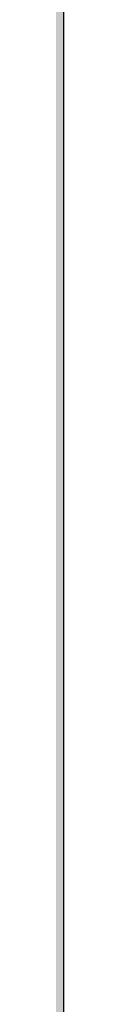
# Model space of a CAD drawing. Units: inches. Extents: x 2091 to 2899, y 967 to 2217.
# Tile 66 of 256: x 2212.1436 to 2212.1443, y 1100.4988 to 1101.1654. Entities that reach past the tile are written whole.
import ezdxf

# ---------------------------------------------------------------- set-up
doc = ezdxf.new("R2010")
doc.units = ezdxf.units.IN
doc.layers.add('A-ANNO-DIMS', color=2, linetype='Continuous', lineweight=18)
doc.layers.add('A-WALL-PATT', color=141, linetype='Continuous', lineweight=13, true_color=0xadddf7)
doc.styles.get("Standard").update_dxf_attribs({"font": 'arial.ttf'})
doc.dimstyles.new('ISO-25', dxfattribs={"dimtxt": 4, "dimasz": 4, "dimexe": 1.25, "dimexo": 0.625, "dimtad": 1, "dimdec": 0, "dimlunit": 3, "dimtxsty": 'Standard', "dimcen": 2.5, "dimadec": 0, "dimazin": 0, "dimtfac": 1, "dimtdec": 0, "dimtmove": 0, "dimatfit": 3, "dimfxl": 1, "dimarcsym": 0})

# ---------------------------------------------------------------- blocks, each defined once
blk = doc.blocks.new('*D71')
at = {"layer": 'A-ANNO-DIMS', "color": 0, "lineweight": -2, "transparency": 16777216}
for p, q in [((2212.1436, 1351.29406), (2212.1436, 969.4643)), ((2452.1436, 1351.29406), (2452.1436, 969.4643)), ((2216.1436, 970.7143), (2448.1436, 970.7143))]:
    blk.add_line(p, q, dxfattribs=at)
at = {"layer": 'A-ANNO-DIMS', "color": 0, "transparency": 16777216}
for points in [[(2216.1436, 971.38097), (2216.1436, 970.04764), (2212.1436, 970.7143)], [(2448.1436, 971.38097), (2448.1436, 970.04764), (2452.1436, 970.7143)]]:
    blk.add_solid(points, dxfattribs=at)
at = {"layer": 'Defpoints', "color": 0, "transparency": 16777216}
for p in [(2212.1436, 1351.91906), (2452.1436, 1351.91906), (2452.1436, 970.7143)]:
    blk.add_point(p, dxfattribs=at)
at = {"layer": 'A-ANNO-DIMS', "color": 0, "transparency": 16777216, "insert": (2332.1436, 973.38159), "char_height": 4, "attachment_point": 5}
blk.add_mtext('20\'-0"', dxfattribs=at)
blk = doc.blocks.new('*D75')
at = {"layer": 'A-ANNO-DIMS', "color": 0, "lineweight": -2, "transparency": 16777216}
for p, q in [((2212.1436, 1274.79406), (2212.1436, 969.4643)), ((2308.1436, 1274.79406), (2308.1436, 969.4643)), ((2216.1436, 970.7143), (2304.1436, 970.7143))]:
    blk.add_line(p, q, dxfattribs=at)
at = {"layer": 'A-ANNO-DIMS', "color": 0, "transparency": 16777216}
for points in [[(2216.1436, 971.38097), (2216.1436, 970.04764), (2212.1436, 970.7143)], [(2304.1436, 971.38097), (2304.1436, 970.04764), (2308.1436, 970.7143)]]:
    blk.add_solid(points, dxfattribs=at)
at = {"layer": 'Defpoints', "color": 0, "transparency": 16777216}
for p in [(2212.1436, 1275.41906), (2308.1436, 1275.41906), (2308.1436, 970.7143)]:
    blk.add_point(p, dxfattribs=at)
at = {"layer": 'A-ANNO-DIMS', "color": 0, "transparency": 16777216, "insert": (2260.1436, 973.38159), "char_height": 4, "attachment_point": 5}
blk.add_mtext('8\'-0"', dxfattribs=at)
blk = doc.blocks.new('*D91')
at = {"layer": 'A-ANNO-DIMS', "color": 0, "lineweight": -2, "transparency": 16777216}
for p, q in [((2211.65063, 1152.24706), (2098.31133, 1152.24706)), ((2099.56133, 1103.91906), (2099.56133, 1148.24706)), ((2211.5186, 1099.91906), (2098.31133, 1099.91906))]:
    blk.add_line(p, q, dxfattribs=at)
at = {"layer": 'A-ANNO-DIMS', "color": 0, "transparency": 16777216}
for points in [[(2098.89467, 1148.24706), (2100.228, 1148.24706), (2099.56133, 1152.24706)], [(2098.89467, 1103.91906), (2100.228, 1103.91906), (2099.56133, 1099.91906)]]:
    blk.add_solid(points, dxfattribs=at)
at = {"layer": 'Defpoints', "color": 0, "transparency": 16777216}
for p in [(2099.56133, 1152.24706), (2212.27563, 1152.24706), (2212.1436, 1099.91906)]:
    blk.add_point(p, dxfattribs=at)
at = {"layer": 'A-ANNO-DIMS', "color": 0, "transparency": 16777216, "insert": (2096.86812, 1126.08306), "char_height": 4, "attachment_point": 5, "rotation": 90}
blk.add_mtext('4\'-4 1/2"', dxfattribs=at)

msp = doc.modelspace()

# ---------------------------------------------------------------- hatches: boundary and pattern name
at = {"layer": 'A-WALL-PATT'}
h = msp.add_hatch(color=256, dxfattribs=at)
h.dxf.hatch_style = 1
h.paths.add_polyline_path([(2803.1436, 2050.91906), (2203.1436, 2050.91906), (2203.1436, 1090.91906), (2803.1436, 1090.91906)])
h.paths.add_polyline_path([(2635.79885, 1147.54046), (2674.52405, 1147.54046, 0.376086), (2678.52967, 1152.8802), (2678.52967, 1159.55647, 0.333335), (2674.52432, 1163.56185), (2674.52432, 1163.56185), (2674.52432, 1192.93439), (2635.80597, 1192.93439), (2597.08762, 1192.93439), (2597.08762, 1163.56185, 0.333335), (2593.08228, 1159.55647), (2593.08228, 1152.8802, 0.376086), (2597.08789, 1147.54046)], flags=0)
h.paths.add_polyline_path([(2436.01043, 1278.24078, 0.000483), (2435.95264, 1278.21503, -0.001328), (2435.93563, 1278.11169, -0.001711), (2436.11644, 1278.04076, 0.002185)], flags=0)
h.paths.add_polyline_path([(2794.1436, 1143.41906), (2794.1436, 1347.41906), (2543.37017, 1347.41906), (2543.37017, 1351.91906), (2794.1436, 1351.91906), (2794.1436, 1392.71355), (2793.9474, 1392.71355), (2793.9474, 1473.5369), (2794.1436, 1473.5369), (2794.1436, 1531.91906), (2650.1436, 1531.91906), (2650.1436, 1536.41906), (2794.1436, 1536.41906), (2794.1436, 1692.41906), (2609.37561, 1692.41906), (2609.37561, 1644.41906), (2604.87561, 1644.41906), (2604.87561, 1744.91906), (2609.37561, 1744.91906), (2609.37561, 1696.91906), (2794.1436, 1696.91906), (2794.1436, 1780.91906), (2609.6436, 1780.91906), (2493.87561, 1780.91906), (2493.87561, 1785.41906), (2609.6436, 1785.41906), (2794.1436, 1785.41906), (2794.1436, 1847.93882), (2793.95122, 1847.93882), (2793.95122, 1928.76217), (2794.1436, 1928.76217), (2794.1436, 1941.41906), (2614.1436, 1941.41906), (2614.1436, 1821.41906), (2609.6436, 1821.41906), (2609.6436, 1941.41906), (2392.1436, 1941.41906), (2392.1436, 1819.91906), (2387.6436, 1819.91906), (2387.6436, 1941.41906), (2212.1436, 1941.41906), (2212.1436, 1783.91906), (2392.1436, 1783.91906), (2392.1436, 1780.91906), (2212.1436, 1780.91906), (2212.1436, 1629.41906), (2387.6436, 1629.41906), (2387.6436, 1744.91906), (2392.1436, 1744.91906), (2392.1436, 1627.91906), (2317.1436, 1627.91906), (2317.1436, 1551.41906), (2317.1436, 1536.41906), (2459.38359, 1536.41906), (2459.38359, 1602.39648), (2463.88359, 1602.39648), (2463.88359, 1531.91906), (2456.6436, 1531.91906), (2456.6436, 1529.91906), (2452.1436, 1529.91906), (2452.1436, 1531.91906), (2312.6436, 1531.91906), (2312.6436, 1551.41906), (2306.1436, 1551.41906), (2306.1436, 1555.91906), (2308.1436, 1555.91906), (2308.1436, 1551.41906), (2312.6436, 1551.41906), (2312.6436, 1627.91906), (2212.1436, 1627.91906), (2212.1436, 1555.91906), (2270.1436, 1555.91906), (2270.1436, 1551.41906), (2212.1436, 1551.41906), (2212.1436, 1351.91906), (2272.1436, 1351.91906), (2272.1436, 1347.41906), (2212.1436, 1347.41906), (2212.1436, 1275.41906), (2308.1436, 1275.41906), (2308.1436, 1351.91906), (2452.1436, 1351.91906), (2452.1436, 1493.91906), (2456.6436, 1493.91906), (2456.6436, 1347.41906), (2312.6436, 1347.41906), (2312.6436, 1270.91906), (2212.1436, 1270.91906), (2212.1436, 1099.91906), (2281.23752, 1099.91906), (2282.87104, 1110.9138), (2282.00834, 1116.9966), (2278.55774, 1121.4204), (2268.20564, 1128.0562), (2272.08764, 1128.0562), (2273.81294, 1131.927), (2279.42034, 1134.6919), (2285.02784, 1135.2449), (2287.61584, 1137.4568), (2288.04714, 1138.0098), (2289.34114, 1140.7747), (2291.06654, 1139.6687), (2292.36054, 1135.2449), (2295.37984, 1136.9038), (2296.24254, 1135.7979), (2297.10524, 1133.033), (2300.12464, 1138.0098), (2303.14394, 1138.0098), (2304.43794, 1135.7979), (2303.14394, 1133.586), (2306.59464, 1134.6919), (2307.88874, 1133.033), (2310.90804, 1135.2449), (2313.92744, 1134.1389), (2315.62686, 1132.4271), (2308.32004, 1117.5496), (2290.20384, 1109.8079), (2288.90984, 1103.1721), (2289.27231, 1099.91906), (2434.91823, 1099.91906), (2431.59323, 1124.78806), (2429.93023, 1169.55306), (2430.92718, 1240.51969), (2435.65893, 1238.18613), (2437.13523, 1196.55406), (2438.79823, 1143.97306), (2442.67823, 1111.99806), (2446.55823, 1099.91906), (2794.1436, 1099.91906), (2794.1436, 1138.91906), (2548.03245, 1138.91906), (2548.03245, 1143.41906), (2548.03245, 1148.81906), (2546.66846, 1148.03156), (2528.68569, 1179.17862, 0.256256), (2512.03245, 1148.81906), (2512.03245, 1143.41906), (2512.03245, 1138.91906), (2507.53245, 1138.91906), (2507.53245, 1143.41906), (2507.53245, 1148.81906, 0.256256), (2490.8792, 1179.17862), (2472.89644, 1148.03156), (2471.53245, 1148.81906), (2471.53245, 1143.41906), (2467.03245, 1143.41906), (2467.03245, 1269.94579, 0.039061), (2460.90999, 1273.58006), (2467.03245, 1273.58006), (2467.03245, 1286.32536, 0.014511), (2465.21619, 1286.76191), (2467.03245, 1287.05258), (2467.03245, 1323.41906), (2471.53245, 1323.41906), (2471.53245, 1148.81906), (2489.53245, 1179.99597), (2490.89644, 1179.20847), (2490.8792, 1179.17862, -0.256256), (2507.53245, 1148.81906), (2507.53245, 1143.41906), (2512.03245, 1143.41906), (2512.03245, 1148.81906, -0.256256), (2528.68569, 1179.17862), (2528.66846, 1179.20847), (2530.03245, 1179.99597), (2548.03245, 1148.81906), (2548.03245, 1143.41906)], flags=16)
h.paths.add_polyline_path([(2607.76855, 1200.94508), (2607.76855, 1265.03063), (2597.08762, 1281.05201), (2619.78459, 1281.05201), (2627.79528, 1337.12686), (2635.79885, 1337.12686), (2643.81666, 1337.12686), (2651.82736, 1281.05201), (2674.52432, 1281.05201), (2663.8434, 1265.03063), (2663.8434, 1200.94508), (2635.80597, 1200.94508)], flags=0)
edge = h.paths.add_edge_path(flags=0)
edge.add_ellipse((13303.89622, 1272.99872), major_axis=(-10595.31304, 0), ratio=0.84230387009, start_angle=0.628237219, end_angle=0.6465541, ccw=False)
edge.add_ellipse((2711.70045, 1156.85268), major_axis=(2.21977, 0), ratio=0.8423039, start_angle=111.53524, end_angle=180.62824, ccw=False)
edge.add_ellipse((13303.15629, 1272.99872), major_axis=(-10593.02631, 0), ratio=0.84230386954, start_angle=0.528271472, end_angle=0.646554097, ccw=False)
edge.add_line((2710.7646, 1175.3333), (2710.12999, 1175.3333))
edge.add_ellipse((2710.12999, 1176.57978), major_axis=(1.47985, 0), ratio=0.8423039, start_angle=180, end_angle=270, ccw=False)
edge.add_line((2708.65014, 1176.57978), (2708.65014, 1200.78291))
edge.add_ellipse((2710.12999, 1200.78291), major_axis=(1.47985, 0), ratio=0.8423039, start_angle=90, end_angle=180, ccw=False)
edge.add_line((2710.12999, 1202.02939), (2710.46508, 1202.02939))
edge.add_ellipse((13303.15629, 1272.99872), major_axis=(-10593.02631, 0), ratio=0.84230386954, start_angle=-0.090229089, end_angle=0.383866779, ccw=False)
edge.add_ellipse((2710.12999, 1290.92703), major_axis=(-1.47985, 0), ratio=0.8423039, start_angle=0, end_angle=90, ccw=False)
edge.add_line((2708.65014, 1290.92703), (2708.65014, 1315.13017))
edge.add_ellipse((2710.12999, 1315.13017), major_axis=(-1.47985, 0), ratio=0.8423039, start_angle=-90, end_angle=0, ccw=False)
edge.add_line((2710.12999, 1316.37665), (2710.70631, 1316.37665))
edge.add_ellipse((3238.40172, 1296.28957), major_axis=(528.234, 0), ratio=0.84230387, start_angle=176.3495724, end_angle=177.8200497, ccw=False)
edge.add_ellipse((2775.06304, 1071.4507), major_axis=(313.30776, 0), ratio=0.84230387, start_angle=102.1259656, end_angle=103.780529, ccw=False)
edge.add_ellipse((2775.06304, 1078.3057), major_axis=(-305.30289, 0), ratio=0.84230387, start_angle=-79.790461, end_angle=-77.5553727, ccw=False)
edge.add_ellipse((2695.14177, 1541.97538), major_axis=(-250.96022, 0), ratio=0.84230387, start_angle=99.256566, end_angle=102.5549326)
edge.add_line((2741.41033, 1334.21426), (2747.13255, 1337.37848))
edge.add_ellipse((2747.53862, 1336.85748), major_axis=(-0.73992, 0), ratio=0.842304, start_angle=270, end_angle=307.93313, ccw=False)
edge.add_ellipse((2747.53862, 1336.85748), major_axis=(-0.73992, 0), ratio=0.842304, start_angle=232.06687, end_angle=270, ccw=False)
edge.add_line((2747.94469, 1337.37848), (2753.66691, 1334.21426))
edge.add_ellipse((2799.93547, 1541.97538), major_axis=(250.96022, 0), ratio=0.84230387, start_angle=257.4450674, end_angle=260.743434)
edge.add_ellipse((2720.01419, 1078.3057), major_axis=(305.30289, 0), ratio=0.84230387, start_angle=77.5553727, end_angle=79.790461, ccw=False)
edge.add_ellipse((2720.01419, 1071.4507), major_axis=(-313.30776, 0), ratio=0.84230387, start_angle=256.219471, end_angle=257.8740344, ccw=False)
edge.add_ellipse((2256.67551, 1296.28957), major_axis=(-528.234, 0), ratio=0.84230387, start_angle=182.1799503, end_angle=183.6504276, ccw=False)
edge.add_line((2784.37092, 1316.37665), (2784.94725, 1316.37665))
edge.add_ellipse((2784.94725, 1315.13017), major_axis=(1.47985, 0), ratio=0.8423039, start_angle=0, end_angle=90, ccw=False)
edge.add_line((2786.42709, 1315.13017), (2786.42709, 1290.92703))
edge.add_ellipse((2784.94725, 1290.92703), major_axis=(1.47985, 0), ratio=0.8423039, start_angle=270, end_angle=360, ccw=False)
edge.add_ellipse((-7808.07906, 1272.99872), major_axis=(10593.02631, 0), ratio=0.84230386954, start_angle=-0.383866779, end_angle=0.090229089, ccw=False)
edge.add_line((2784.61216, 1202.02939), (2784.94725, 1202.02939))
edge.add_ellipse((2784.94725, 1200.78291), major_axis=(1.47985, 0), ratio=0.8423039, start_angle=0, end_angle=90, ccw=False)
edge.add_line((2786.42709, 1200.78291), (2786.42709, 1176.57978))
edge.add_ellipse((2784.94725, 1176.57978), major_axis=(-1.47985, 0), ratio=0.8423039, start_angle=90, end_angle=180, ccw=False)
edge.add_line((2784.94725, 1175.3333), (2784.31264, 1175.3333))
edge.add_ellipse((-7808.07906, 1272.99872), major_axis=(10593.02631, 0), ratio=0.84230386954, start_angle=-0.618643196, end_angle=-0.528271472, ccw=False)
edge.add_ellipse((2783.37678, 1156.85268), major_axis=(-2.21977, 0), ratio=0.8423039, start_angle=179.37176, end_angle=248.46476, ccw=False)
edge.add_ellipse((-7808.81898, 1272.99872), major_axis=(-10595.31304, 0), ratio=0.84230386576, start_angle=179.353445923, end_angle=179.371762803, ccw=False)
edge.add_ellipse((2780.2973, 1153.50079), major_axis=(-5.24643, 0), ratio=0.8423039, start_angle=90, end_angle=179.35345, ccw=False)
edge.add_line((2780.2973, 1149.08171), (2714.77993, 1149.08171))
edge.add_ellipse((2714.77993, 1153.50079), major_axis=(5.24643, 0), ratio=0.8423039, start_angle=180.64655, end_angle=270, ccw=False)
edge = h.paths.add_edge_path(flags=0)
edge.add_line((2718.18737, 1151.00783), (2718.18737, 1170.47236))
edge.add_ellipse((2721.14706, 1170.47236), major_axis=(-2.95969, 0), ratio=0.8423039, start_angle=-90, end_angle=0, ccw=False)
edge.add_line((2721.14706, 1172.96532), (2773.93017, 1172.96532))
edge.add_ellipse((2773.93017, 1170.47236), major_axis=(-2.95969, 0), ratio=0.8423039, start_angle=180, end_angle=270, ccw=False)
edge.add_line((2776.88987, 1170.47236), (2776.88987, 1151.00783))
edge.add_line((2776.88987, 1151.00783), (2718.18737, 1151.00783))
edge = h.paths.add_edge_path(flags=0)
edge.add_line((2718.18737, 1180.23415), (2718.18737, 1199.05783))
edge.add_ellipse((2747.53862, 1320.39864), major_axis=(147.01792, 0), ratio=0.84230387, start_angle=256.4018653, end_angle=283.5981347)
edge.add_line((2776.88987, 1199.05783), (2776.88987, 1180.23415))
edge.add_ellipse((2747.53862, 1301.57496), major_axis=(147.01792, 0), ratio=0.84230387, start_angle=256.4018653, end_angle=283.5981347, ccw=False)
edge = h.paths.add_edge_path(flags=0)
edge.add_ellipse((13303.15629, 1272.99872), major_axis=(-10591.54646, 0), ratio=0.84230386955, start_angle=0.055594314, end_angle=0.377764194, ccw=False)
edge.add_line((2711.61686, 1262.72171), (2715.66741, 1249.4954))
edge.add_ellipse((6413.89196, 1241.69192), major_axis=(-3698.23616, 0), ratio=0.8423038695, start_angle=-0.12089737, end_angle=0.36407635)
edge.add_line((2715.76104, 1218.19245), (2711.93431, 1203.16736))
edge = h.paths.add_edge_path(flags=0)
edge.add_line((2718.18737, 1251.07457), (2716.00249, 1267.45044))
edge.add_ellipse((2742.15117, 1202.18954), major_axis=(81.77258, 0), ratio=0.84230387, start_angle=94.277421, end_angle=111.8349538, ccw=False)
edge.add_line((2737.00975, 1270.93063), (2758.06748, 1270.93063))
edge.add_ellipse((2752.92606, 1202.18954), major_axis=(81.77258, 0), ratio=0.84230387, start_angle=68.1650462, end_angle=85.722579, ccw=False)
edge.add_line((2779.07475, 1267.45044), (2776.88987, 1251.07457))
edge.add_ellipse((2750.33806, 1187.88536), major_axis=(79.57966, 0), ratio=0.84230387, start_angle=67.2080851, end_angle=85.1299304)
edge.add_line((2756.03466, 1254.74366), (2739.04258, 1254.74366))
edge.add_ellipse((2744.73917, 1187.88536), major_axis=(79.57966, 0), ratio=0.84230387, start_angle=94.8700696, end_angle=112.7919149)
edge = h.paths.add_edge_path(flags=0)
edge.add_line((2783.14293, 1203.16736), (2779.31619, 1218.19245))
edge.add_ellipse((-918.81473, 1241.69192), major_axis=(3698.23616, 0), ratio=0.8423038695, start_angle=-0.36407635, end_angle=0.12089737)
edge.add_line((2779.40983, 1249.4954), (2783.46037, 1262.72171))
edge.add_ellipse((-7808.07906, 1272.99872), major_axis=(-10591.54646, 0), ratio=0.84230386954, start_angle=179.622235806, end_angle=179.944405687, ccw=False)
edge = h.paths.add_edge_path(flags=0)
edge.add_ellipse((2734.20089, 1286.69044), major_axis=(-0.35661, 6.34008), ratio=0.6038336, start_angle=89.002014, end_angle=253.657408, ccw=False)
edge.add_line((2730.369, 1286.54181), (2730.369, 1301.35198))
edge.add_line((2730.369, 1301.35198), (2735.91331, 1305.2148))
edge.add_ellipse((2736.38492, 1304.73456), major_axis=(0.73992, 0), ratio=0.842304, start_angle=90, end_angle=134.48021, ccw=False)
edge.add_line((2736.38492, 1305.3578), (2738.03278, 1305.3578))
edge.add_line((2738.03278, 1305.3578), (2738.03278, 1307.70793))
edge.add_ellipse((2794.20164, 1307.70793), major_axis=(56.16886, 0), ratio=0.84230387, start_angle=150.56143, end_angle=180, ccw=False)
edge.add_ellipse((2700.87559, 1307.70793), major_axis=(-56.16886, 0), ratio=0.84230387, start_angle=180, end_angle=209.43857, ccw=False)
edge.add_line((2757.04445, 1307.70793), (2757.04445, 1305.3578))
edge.add_line((2757.04445, 1305.3578), (2758.69232, 1305.3578))
edge.add_ellipse((2758.69232, 1304.73456), major_axis=(-0.73992, 0), ratio=0.842304, start_angle=225.51979, end_angle=270, ccw=False)
edge.add_line((2759.16392, 1305.2148), (2764.70823, 1301.35198))
edge.add_line((2764.70823, 1301.35198), (2764.70823, 1286.54181))
edge.add_ellipse((2760.87634, 1286.69044), major_axis=(0.35661, 6.34008), ratio=0.6038336, start_angle=106.342592, end_angle=270.997986, ccw=False)
edge.add_line((2757.04445, 1285.79709), (2757.04445, 1307.70793))
edge.add_ellipse((2700.87559, 1307.70793), major_axis=(-56.16886, 0), ratio=0.84230387, start_angle=180, end_angle=209.43857)
edge.add_ellipse((2794.20164, 1307.70793), major_axis=(56.16886, 0), ratio=0.84230387, start_angle=150.56143, end_angle=180)
edge.add_line((2738.03278, 1307.70793), (2738.03278, 1285.79709))
h.paths.add_polyline_path([(2417.81227, 1104.4497), (2413.49227, 1102.5297), (2410.61227, 1103.9697), (2409.17227, 1106.3697), (2407.25227, 1107.3297), (2406.29227, 1109.7297), (2405.33227, 1114.0497), (2405.33227, 1117.8897), (2406.29227, 1120.1297), (2407.25227, 1119.8097), (2408.84832, 1118.32766), (2410.17395, 1119.42417), (2410.21127, 1120.4057), (2411.04073, 1121.41905), (2410.69927, 1119.8587), (2410.17395, 1119.42417), (2410.08845, 1117.17611), (2411.13284, 1116.20632), (2413.97227, 1119.3297), (2416.85227, 1120.7697), (2416.86972, 1120.79878), (2417.03507, 1119.40512), (2417.89621, 1118.14338), (2418.29227, 1118.3697), (2419.54445, 1120.03927), (2419.36092, 1118.38749), (2419.03211, 1119.35615), (2418.39894, 1118.51193), (2419.25227, 1114.5297), (2418.79409, 1107.19879)], flags=0)
h.paths.add_polyline_path([(2508.87017, 1347.41906), (2508.37017, 1347.41906), (2508.37017, 1351.91906), (2508.87017, 1351.91906)], flags=0)
h.paths.add_polyline_path([(2473.37017, 1347.41906), (2472.37017, 1347.41906), (2467.87017, 1347.41906), (2467.87017, 1455.41906), (2472.37017, 1455.41906), (2472.37017, 1352.41906), (2473.37017, 1352.41906)], flags=0)
h.paths.add_polyline_path([(2352.10624, 1217.4462), (2349.22624, 1218.8862), (2347.78624, 1221.2862), (2345.86624, 1222.2462), (2344.90624, 1224.6462), (2343.94624, 1228.9662), (2343.94624, 1232.8062), (2344.90624, 1235.0462), (2345.86624, 1234.7262), (2347.46229, 1233.24415), (2348.78792, 1234.34066), (2348.82524, 1235.3222), (2349.6547, 1236.33555), (2349.31324, 1234.7752), (2348.78792, 1234.34066), (2348.70242, 1232.0926), (2349.74681, 1231.12282), (2352.58624, 1234.2462), (2355.46624, 1235.6862), (2355.48369, 1235.71528), (2355.64904, 1234.32161), (2356.51018, 1233.05988), (2356.90624, 1233.2862), (2358.15842, 1234.95576), (2357.97489, 1233.30398), (2357.64608, 1234.27264), (2357.01291, 1233.42842), (2357.86624, 1229.4462), (2357.40806, 1222.11529), (2356.42624, 1219.3662)], flags=0)
h.paths.add_polyline_path([(2348.2968, 1112.22442), (2347.0138, 1112.31042), (2345.5298, 1114.12742), (2345.7318, 1115.85842), (2346.8118, 1116.98242), (2346.8118, 1114.64642), (2345.8668, 1114.21442), (2346.8798, 1114.30042)], flags=0)
h.paths.add_polyline_path([(2347.0138, 1110.92642), (2346.2718, 1110.49342), (2346.6098, 1111.18642)], flags=0)
h.paths.add_polyline_path([(2345.8668, 1118.19442), (2345.5298, 1117.32942), (2343.7078, 1118.02142), (2344.3828, 1118.62642)], flags=0)
h.paths.add_polyline_path([(2346.6768, 1109.28242), (2346.0698, 1108.07142), (2345.8668, 1110.06142)], flags=0)
h.paths.add_polyline_path([(2345.0568, 1119.75142), (2343.6398, 1119.75142), (2343.9778, 1121.13542)], flags=0)
h.paths.add_polyline_path([(2345.2598, 1116.55042), (2345.1248, 1115.85842), (2344.9218, 1115.68542), (2344.7198, 1116.37742)], flags=0)
h.paths.add_polyline_path([(2345.6648, 1112.31042), (2345.4618, 1111.53242), (2344.0448, 1111.96442), (2344.6518, 1112.57042)], flags=0)
h.paths.add_polyline_path([(2345.1918, 1113.34942), (2344.4498, 1113.86842), (2344.7198, 1114.38742)], flags=0)
h.paths.add_polyline_path([(2344.6518, 1116.80942), (2344.1798, 1115.68542), (2344.6518, 1115.33942), (2343.9098, 1114.90642), (2343.0328, 1115.94442), (2343.6398, 1116.46342)], flags=0)
h.paths.add_polyline_path([(2345.8668, 1106.68642), (2344.9898, 1105.56242), (2344.5168, 1106.60042)], flags=0)
h.paths.add_polyline_path([(2344.8548, 1110.06142), (2344.5168, 1109.28242), (2344.1128, 1109.71542)], flags=0)
h.paths.add_polyline_path([(2344.0448, 1113.52242), (2343.4378, 1113.08942), (2342.7628, 1113.95442)], flags=0)
h.paths.add_polyline_path([(2344.3148, 1111.01242), (2342.9648, 1110.32042), (2342.9648, 1111.09942)], flags=0)
h.paths.add_polyline_path([(2345.1248, 1104.69742), (2344.5848, 1103.74542), (2344.4498, 1104.26442)], flags=0)
h.paths.add_polyline_path([(2342.8298, 1121.22242), (2341.7498, 1120.53042), (2340.5358, 1121.04942), (2340.1308, 1121.82842), (2340.6708, 1122.95242), (2341.1428, 1121.82842), (2341.6148, 1122.00142)], flags=0)
h.paths.add_polyline_path([(2342.9648, 1119.75142), (2343.0328, 1118.45342), (2342.0878, 1118.02142), (2342.0198, 1119.49142)], flags=0)
h.paths.add_polyline_path([(2342.6948, 1116.89642), (2341.9528, 1116.63642), (2342.0198, 1117.32942)], flags=0)
h.paths.add_polyline_path([(2343.0328, 1112.22442), (2342.0198, 1111.79142), (2341.5478, 1112.22442), (2342.3578, 1113.34942)], flags=0)
h.paths.add_polyline_path([(2343.7748, 1104.43742), (2342.6278, 1102.88042), (2342.6948, 1104.61042), (2343.4378, 1105.12942)], flags=0)
h.paths.add_polyline_path([(2342.0198, 1115.07942), (2340.8058, 1115.51242), (2340.9408, 1116.37742)], flags=0)
h.paths.add_polyline_path([(2341.4808, 1120.09742), (2341.4808, 1119.40542), (2341.0758, 1119.57842), (2341.1428, 1120.09742)], flags=0)
h.paths.add_polyline_path([(2341.8178, 1114.47342), (2340.9408, 1113.08942), (2340.8058, 1114.56042)], flags=0)
h.paths.add_polyline_path([(2341.1428, 1118.54042), (2340.9408, 1116.98242), (2339.0508, 1117.67542), (2339.0508, 1118.62642)], flags=0)
h.paths.add_polyline_path([(2342.6948, 1101.66842), (2341.9528, 1101.84142), (2342.5598, 1102.36142)], flags=0)
h.paths.add_polyline_path([(2340.3328, 1119.66542), (2338.4438, 1119.57842), (2337.9038, 1120.35742), (2339.6578, 1120.61642)], flags=0)
h.paths.add_polyline_path([(2340.3328, 1115.33942), (2340.0628, 1113.69542), (2339.3878, 1115.33942)], flags=0)
h.paths.add_polyline_path([(2341.8178, 1103.83142), (2341.5478, 1102.88042), (2341.1428, 1103.65842)], flags=0)
h.paths.add_polyline_path([(2339.0508, 1122.86642), (2337.2958, 1121.82842), (2337.0938, 1123.12542), (2337.7688, 1123.81842)], flags=0)
h.paths.add_polyline_path([(2339.1178, 1121.74142), (2338.8478, 1121.22242), (2338.1738, 1121.04942), (2338.3758, 1121.56842)], flags=0)
h.paths.add_polyline_path([(2339.1858, 1119.31942), (2338.6458, 1118.71342), (2338.2408, 1118.10742), (2338.2408, 1118.88642)], flags=0)
h.paths.add_polyline_path([(2341.1428, 1101.92842), (2340.6028, 1101.23642), (2340.0628, 1101.84142), (2340.6028, 1102.36142)], flags=0)
h.paths.add_polyline_path([(2337.6338, 1117.76142), (2336.6208, 1118.28042), (2337.2958, 1118.97242)], flags=0)
h.paths.add_polyline_path([(2336.8238, 1119.57842), (2334.7988, 1118.97242), (2335.2038, 1120.35742), (2336.5538, 1120.87642)], flags=0)
h.paths.add_polyline_path([(2339.1178, 1100.45742), (2337.3638, 1100.54342), (2336.7558, 1101.23642)], flags=0)
h.paths.add_polyline_path([(2336.3508, 1122.43342), (2336.0138, 1121.91442), (2334.9338, 1122.43342), (2334.5288, 1123.47142), (2335.7438, 1122.77942)], flags=0)
h.paths.add_polyline_path([(2334.7318, 1120.87642), (2334.2588, 1120.35742), (2334.0568, 1120.78942), (2334.5968, 1121.30842)], flags=0)
h.paths.add_polyline_path([(2334.4618, 1122.17442), (2332.5718, 1121.30842), (2331.3568, 1122.17442), (2332.0998, 1122.86642)], flags=0)
h.paths.add_polyline_path([(2334.2588, 1118.54042), (2333.3818, 1118.45342), (2333.6518, 1119.31942)], flags=0)
h.paths.add_polyline_path([(2335.5418, 1102.27442), (2334.1918, 1102.62042), (2335.2718, 1103.31242)], flags=0)
h.paths.add_polyline_path([(2332.7068, 1119.66542), (2331.6948, 1120.44342), (2332.5048, 1120.78942)], flags=0)
h.paths.add_polyline_path([(2334.7318, 1101.14942), (2333.5168, 1101.58242), (2333.9888, 1101.75542)], flags=0)
h.paths.add_polyline_path([(2332.6398, 1116.63642), (2331.0868, 1116.29042), (2331.9648, 1118.19442)], flags=0)
h.paths.add_polyline_path([(2330.7498, 1121.56842), (2330.2768, 1120.27042), (2328.5228, 1119.31942), (2328.9948, 1121.04942)], flags=0)
h.paths.add_polyline_path([(2330.7498, 1118.62642), (2330.0078, 1117.50242), (2329.8728, 1118.02142)], flags=0)
h.paths.add_polyline_path([(2332.0998, 1102.36142), (2330.5468, 1102.01442), (2331.6948, 1102.96642)], flags=0)
h.paths.add_polyline_path([(2329.5348, 1113.60842), (2329.0628, 1112.31042), (2328.5898, 1113.34942)], flags=0)
h.paths.add_polyline_path([(2328.3878, 1117.84842), (2327.5098, 1116.55042), (2327.1728, 1117.76142)], flags=0)
h.paths.add_polyline_path([(2329.7378, 1106.51342), (2329.5348, 1105.30242), (2328.2528, 1106.08142)], flags=0)
h.paths.add_polyline_path([(2328.6578, 1114.38742), (2328.0498, 1114.12742), (2328.3198, 1114.90642)], flags=0)
h.paths.add_polyline_path([(2328.3198, 1112.22442), (2327.1058, 1112.13742), (2326.7008, 1112.65642)], flags=0)
h.paths.add_polyline_path([(2326.9028, 1115.25242), (2326.7008, 1114.12742), (2325.2158, 1113.60842), (2326.0928, 1115.33942)], flags=0)
h.paths.add_polyline_path([(2326.6328, 1108.33042), (2326.0928, 1107.37942), (2325.8908, 1108.50342), (2326.4978, 1109.10942)], flags=0)
h.paths.add_polyline_path([(2615.1436, 1531.91906), (2609.6436, 1531.91906), (2609.6436, 1620.41906), (2614.1436, 1620.41906), (2614.1436, 1536.41906), (2615.1436, 1536.41906)], flags=0)
h.paths.add_polyline_path([(2545.1436, 1563.41906), (2464.1436, 1563.41906), (2464.1436, 1632.41906), (2509.1436, 1632.41906), (2509.1436, 1627.91906), (2509.1436, 1603.91906), (2468.6436, 1603.91906), (2468.6436, 1567.91906), (2540.6436, 1567.91906), (2540.6436, 1591.91906), (2545.1436, 1591.91906)], flags=0)
h.paths.add_polyline_path([(2388.96905, 1549.98573), (2357.43418, 1549.98573), (2357.43418, 1623.36078), (2399.36278, 1623.36078), (2435.68947, 1623.36078), (2435.59255, 1602.55927), (2435.59255, 1602.39648), (2388.96905, 1602.39648)], flags=0)
h.paths.add_polyline_path([(2388.88063, 1555.80915), (2374.90443, 1555.80915), (2374.90443, 1600.57156), (2374.90443, 1615.45765), (2406.35088, 1615.45765), (2406.35088, 1618.93943), (2412.17429, 1615.45765), (2406.35088, 1611.97586), (2406.35088, 1615.45765), (2388.88063, 1615.45765)], flags=0)
h.paths.add_polyline_path([(2568.87561, 1644.41906), (2453.37561, 1644.41906), (2453.37561, 1785.41906), (2457.87561, 1785.41906), (2457.87561, 1648.91906), (2568.87561, 1648.91906)], flags=0)
h.paths.add_polyline_path([(2212.1436, 1945.91906), (2212.1436, 2041.91906), (2794.1436, 2041.91906), (2794.1436, 1945.91906)], flags=16)
h.paths.add_polyline_path([(2271.08273, 1964.31724), (2776.85297, 1964.31724), (2776.85297, 2037.16962), (2271.08273, 2037.16962)], flags=8)
h.paths.add_polyline_path([(2380.64929, 1536.82414), (2461.04081, 1536.82414), (2461.04081, 1554.65259), (2380.64929, 1554.65259)], flags=8)
h.paths.add_polyline_path([(2240.75571, 1609.72545), (2309.18583, 1609.72545), (2309.18583, 1617.6982), (2240.75571, 1617.6982)], flags=8)
h.paths.add_polyline_path([(2212.67726, 1313.5041), (2282.59152, 1313.5041), (2282.59152, 1322.74524), (2212.67726, 1322.74524)], flags=8)
h.paths.add_polyline_path([(2457.11198, 1114.77857), (2558.48158, 1114.77857), (2558.48158, 1142.21968), (2457.11198, 1142.21968)], flags=8)
h.paths.add_polyline_path([(2473.44234, 1273.01007), (2604.64123, 1273.01007), (2604.64123, 1318.34693), (2473.44234, 1318.34693)], flags=8)
h.paths.add_polyline_path([(2638.8763, 1626.97743), (2684.25037, 1627.97674), (2684.03848, 1637.59749), (2638.66442, 1636.59819)], flags=8)
h.paths.add_polyline_path([(2537.59055, 1453.79345), (2628.38955, 1453.79345), (2628.38955, 1475.34481), (2537.59055, 1475.34481)], flags=8)
h.paths.add_polyline_path([(2504.13764, 1714.6324), (2554.64719, 1714.6324), (2554.64719, 1730.23771), (2504.13764, 1730.23771)], flags=8)
h.paths.add_polyline_path([(2487.50118, 1575.65187), (2535.09712, 1575.65187), (2535.09712, 1598.37765), (2487.50118, 1598.37765)], flags=8)
h.paths.add_polyline_path([(2709.0994, 1735.71028), (2740.0166, 1735.71028), (2740.0166, 1749.93764), (2709.0994, 1749.93764)], flags=8)
h.paths.add_polyline_path([(2442.43842, 1792.17166), (2564.72884, 1792.17166), (2564.72884, 1842.00016), (2442.43842, 1842.00016)], flags=8)
h.paths.add_polyline_path([(2655.8158, 1809.64408), (2789.52014, 1806.6938), (2790.08498, 1832.29164), (2656.38064, 1835.24192)], flags=8)
h.paths.add_polyline_path([(2234.8427, 1797.72014), (2368.59285, 1794.76885), (2369.16072, 1820.50413), (2235.41056, 1823.45542)], flags=8)
h.paths.add_polyline_path([(2245.13847, 1644.00633), (2398.42773, 1640.6239), (2398.99484, 1666.32482), (2245.70557, 1669.70725)], flags=8)
h.paths.add_polyline_path([(2306.14285, 1431.16852), (2413.76831, 1428.79369), (2414.33315, 1454.39153), (2306.70768, 1456.76636)], flags=8)
h.paths.add_polyline_path([(2306.83458, 1458.23314), (2393.38048, 1456.32345), (2393.93281, 1481.35436), (2307.38691, 1483.26405)], flags=8)

# ---------------------------------------------------------------- dimensions: what is measured, and where the dimension line sits
at = {"layer": 'A-ANNO-DIMS'}
for base, p1, p2, picture, middle in [((2452.1436, 970.7143), (2212.1436, 1351.91906), (2452.1436, 1351.91906), '*D71', (2332.1436, 973.38159)), ((2308.1436, 970.7143), (2212.1436, 1275.41906), (2308.1436, 1275.41906), '*D75', (2260.1436, 973.38159))]:
    dim = msp.add_linear_dim(base=base, p1=p1, p2=p2, dimstyle='ISO-25', override={"dimdec": 1, "dimlfac": 1, "dimrnd": 0, "dimzin": 1, "dimdsep": 46, "dimlunit": 4, "dimfrac": 2}, dxfattribs=at)
    dim.commit()
    dim.dimension.update_dxf_attribs({"geometry": picture, "text_midpoint": middle})
dim = msp.add_linear_dim(base=(2099.56133, 1152.24706), p1=(2212.1436, 1099.91906), p2=(2212.27563, 1152.24706), angle=90, dimstyle='ISO-25', override={"dimdec": 1, "dimlfac": 1, "dimrnd": 0, "dimzin": 1, "dimdsep": 46, "dimlunit": 4, "dimfrac": 2}, dxfattribs=at)
dim.commit()
dim.dimension.update_dxf_attribs({"geometry": '*D91', "text_midpoint": (2096.86812, 1126.08306)})

doc.saveas('drawing.dxf')
